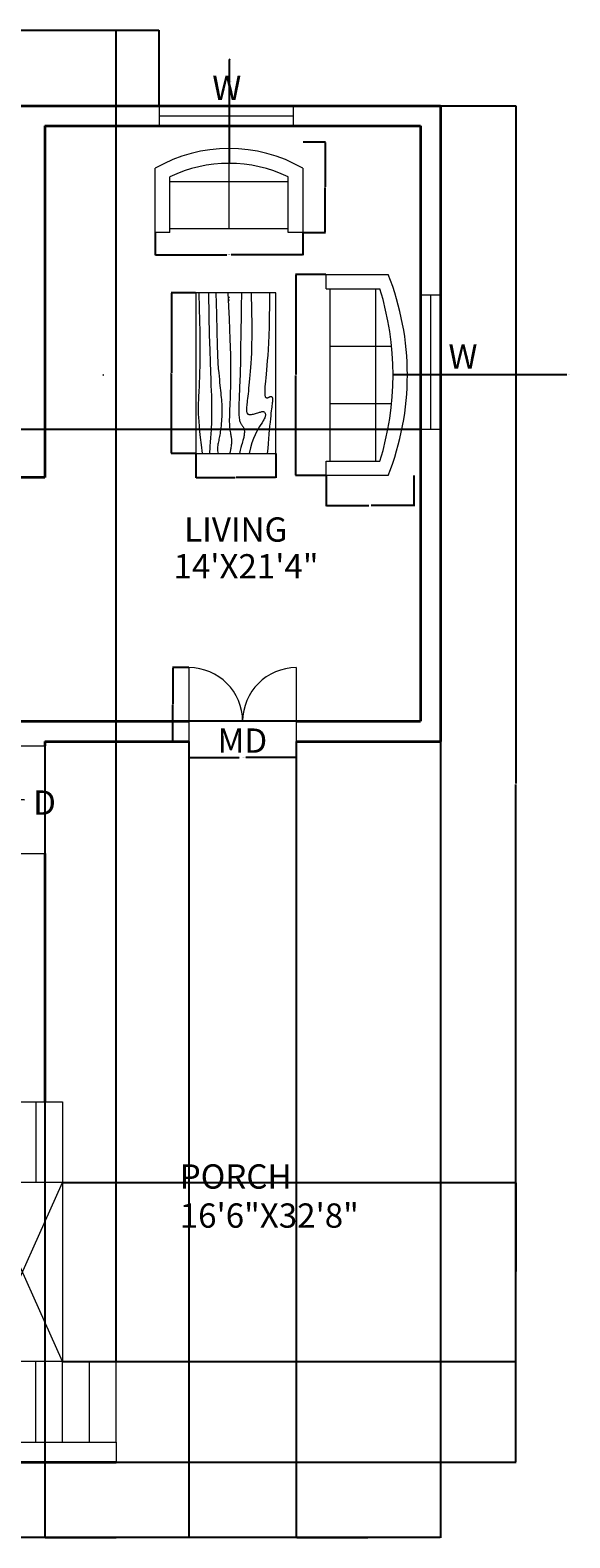
# Model space of a CAD drawing. Units: feet. Extents: x 1681 to 2398, y 1737 to 2411.
# Tile 4 of 4: x 2156 to 2398, y 1737 to 2411. Entities that reach past the tile are written whole.
import ezdxf

# ---------------------------------------------------------------- set-up
doc = ezdxf.new("R2010")
doc.units = ezdxf.units.FT
for name, color, linetype, lineweight in [('A-ANNO-DIMS', 2, 'Continuous', 18), ('A-ANNO-TEXT', 7, 'Continuous', 18), ('A-AREA-IDEN', 7, 'Continuous', 18), ('A-DOOR', 3, 'Continuous', 18), ('A-FLOR', 7, 'Continuous', 25), ('A-FLOR-STRS', 7, 'Continuous', 18), ('A-FURN', 8, 'Continuous', 13), ('A-GLAZ', 4, 'Continuous', 18), ('A-WALL', 7, 'Continuous', 35)]:
    doc.layers.add(name, color=color, linetype=linetype, lineweight=lineweight)
doc.styles.get("Standard").update_dxf_attribs({"font": 'arial.ttf'})
doc.dimstyles.get("Standard").update_dxf_attribs({"dimtxt": 0.18, "dimasz": 0.18, "dimexe": 0.18, "dimexo": 0.0625, "dimgap": 0.09, "dimtad": 0, "dimtih": 1, "dimtoh": 1, "dimdec": 4, "dimzin": 0, "dimdsep": 46, "dimtxsty": 'Standard', "dimcen": 0.09, "dimadec": 0, "dimazin": 0, "dimtfac": 1, "dimtdec": 4, "dimtofl": 0, "dimtmove": 0, "dimatfit": 3, "dimfxl": 1, "dimtolj": 1, "dimtzin": 0, "dimarcsym": 0})

# ---------------------------------------------------------------- blocks, each defined once
blk = doc.blocks.new('Sofa - Roundback 7 ft.')
for p, q in [((-36.000027, -34), (-36.000027, -11.4696)), ((-12.00002, -32.4421), (-12.00003, -6.5971)), ((11.99997, -32.4421), (11.99998, -6.5971)), ((35.99998, -34), (35.99998, -11.4696)), ((-35.999844, -13.3819), (35.9998, -13.3819)), ((-36.000027, -32.4421), (35.99998, -32.4421))]:
    blk.add_line(p, q)
for points in [[(-36.000027, -34), (-42.000027, -34), (-42.000027, -8)], [(41.99998, -8), (41.99998, -34), (35.99998, -34)]]:
    blk.add_lwpolyline(points)
for centre, radius, start, end in [((0, -114.25), 114.25, 68.43141, 111.5686), ((-0.00001, -127.1968), 121.1968, 72.72033, 107.2797)]:
    blk.add_arc(centre, radius, start, end)
blk = doc.blocks.new('Sofa - Roundback Loveseat 5 ft.')
for p, q in [((0, -32.44198), (0, -5.99998)), ((-24, -33.99998), (-24, -11.46958)), ((24.00004, -33.99998), (24.00004, -11.46958)), ((-23.9998, -13.38178), (23.99986, -13.38178)), ((-24, -32.44198), (24.00004, -32.44198))]:
    blk.add_line(p, q)
for points in [[(-24, -33.99998), (-30, -33.99998), (-30, -7.99998)], [(30.00004, -7.99998), (30.00004, -33.99998), (24.00004, -33.99998)]]:
    blk.add_lwpolyline(points)
for centre, radius, start, end in [((0, -60.24998), 60.24998, 60.13715, 119.8628), ((0, -61.38438), 55.38444, 64.32083, 115.6792)]:
    blk.add_arc(centre, radius, start, end)
blk = doc.blocks.new('Table - Rectangular Woodgrain 60 x 30 in.')
for p, q in [((0, 0), (0, -30)), ((60, 0), (0, 0)), ((60, -30), (60, 0)), ((0, -30), (60, -30))]:
    blk.add_line(p, q)
for points in [[(0, -2.4), (4.8155, -2.418), (9.0302, -2.4688), (12.709, -2.5477), (15.9167, -2.65), (18.7181, -2.7711), (21.1781, -2.9063), (23.3616, -3.0508), (25.3333, -3.2), (27.1477, -3.3495), (28.8172, -3.4958), (30.3437, -3.636), (31.7291, -3.7667), (32.9756, -3.8849), (34.0849, -3.9875), (35.059, -4.0714), (35.9, -4.1334), (36.6114, -4.1711), (37.2041, -4.1854), (37.6906, -4.1779), (38.0833, -4.15), (38.3948, -4.1034), (38.6375, -4.0396), (38.8239, -3.9602), (38.9666, -3.8667), (39.0764, -3.7608), (39.1573, -3.6448), (39.2116, -3.521), (39.2416, -3.3917), (39.2498, -3.2593), (39.2385, -3.1261), (39.21, -2.9944), (39.1666, -2.8667), (39.111, -2.7447), (39.0468, -2.6281), (38.978, -2.5163), (38.9083, -2.4083), (38.8418, -2.3035), (38.7823, -2.201), (38.7337, -2.1001), (38.7, -2), (38.6844, -1.9003), (38.6875, -1.8021), (38.7094, -1.707), (38.75, -1.6167), (38.8094, -1.5326), (38.8875, -1.4563), (38.9844, -1.3893), (39.1, -1.3333), (39.2351, -1.2896), (39.3937, -1.2583), (39.5804, -1.2396), (39.8, -1.2333), (40.057, -1.2396), (40.3562, -1.2583), (40.7023, -1.2896), (41.1, -1.3333), (41.5547, -1.3895), (42.0755, -1.4573), (42.6721, -1.5361), (43.3542, -1.625), (44.1316, -1.7233), (45.014, -1.8302), (46.0114, -1.9449), (47.1333, -2.0667), (48.3862, -2.1947), (49.7625, -2.3281), (51.2513, -2.4663), (52.8416, -2.6083), (54.5226, -2.7535), (56.2833, -2.9011), (58.1127, -3.0501), (60, -3.2)], [(0, -9.2), (6.5759, -9.0858), (11.9385, -9.0365), (16.2527, -9.0418), (19.6833, -9.0917), (22.3952, -9.1759), (24.5531, -9.2844), (26.322, -9.4069), (27.8666, -9.5333), (29.3241, -9.6553), (30.7203, -9.7719), (32.0532, -9.8837), (33.3208, -9.9917), (34.5213, -10.0965), (35.6526, -10.199), (36.7128, -10.2999), (37.7, -10.4), (38.6129, -10.4996), (39.4531, -10.5969), (40.223, -10.6895), (40.925, -10.775), (41.5613, -10.8512), (42.1344, -10.9156), (42.6465, -10.966), (43.1, -11), (43.4976, -11.0158), (43.8437, -11.0136), (44.143, -10.9942), (44.4, -10.9583), (44.6195, -10.9069), (44.8062, -10.8406), (44.9648, -10.7603), (45.1, -10.6667), (45.2155, -10.5598), (45.3114, -10.4365), (45.3871, -10.2929), (45.4416, -10.125), (45.4743, -9.929), (45.4844, -9.7011), (45.4709, -9.4371), (45.4333, -9.1333), (45.3716, -8.7883), (45.2896, -8.4104), (45.1919, -8.0107), (45.0833, -7.6), (44.9685, -7.1893), (44.8521, -6.7896), (44.7388, -6.4117), (44.6333, -6.0667), (44.54, -5.7628), (44.4614, -5.4979), (44.4001, -5.2675), (44.3583, -5.0667), (44.3384, -4.8909), (44.3427, -4.7354), (44.3736, -4.5956), (44.4333, -4.4667), (44.5236, -4.3453), (44.6427, -4.2333), (44.7884, -4.1339), (44.9583, -4.05), (45.1501, -3.9849), (45.3614, -3.9417), (45.59, -3.9234), (45.8333, -3.9333), (46.0915, -3.9749), (46.3734, -4.0531), (46.6906, -4.1736), (47.0542, -4.3417), (47.4756, -4.5629), (47.9661, -4.8427), (48.5372, -5.1866), (49.2, -5.6), (49.9676, -6.0844), (50.8594, -6.625), (51.8965, -7.2031), (53.1, -7.8), (54.491, -8.3969), (56.0906, -8.975), (57.9199, -9.5156), (60, -10)], [(0, -12.8), (5.1847, -12.9322), (9.6213, -13.0323), (13.3963, -13.1059), (16.5958, -13.1583), (19.3063, -13.1952), (21.614, -13.2219), (23.6054, -13.2439), (25.3666, -13.2667), (26.9728, -13.2947), (28.4531, -13.3281), (29.8256, -13.3663), (31.1083, -13.4083), (32.3191, -13.4535), (33.476, -13.501), (34.597, -13.5501), (35.7, -13.6), (36.7984, -13.6497), (37.8875, -13.6979), (38.9578, -13.743), (40, -13.7833), (41.0047, -13.8174), (41.9625, -13.8438), (42.864, -13.8607), (43.7, -13.8667), (44.4631, -13.8604), (45.1552, -13.8417), (45.7801, -13.8104), (46.3416, -13.7667), (46.8439, -13.7104), (47.2906, -13.6417), (47.6858, -13.5604), (48.0333, -13.4667), (48.3375, -13.3608), (48.6042, -13.2448), (48.8396, -13.121), (49.05, -12.9917), (49.2417, -12.8593), (49.4208, -12.7261), (49.5937, -12.5944), (49.7667, -12.4667), (49.9452, -12.3451), (50.1323, -12.2313), (50.3303, -12.1268), (50.5416, -12.0333), (50.7686, -11.9524), (51.0135, -11.8854), (51.2788, -11.8341), (51.5666, -11.8), (51.8785, -11.7843), (52.2116, -11.7865), (52.562, -11.8059), (52.926, -11.8417), (53.2998, -11.8931), (53.6795, -11.9594), (54.0614, -12.0397), (54.4416, -12.1333), (54.8223, -12.2401), (55.2293, -12.3625), (55.6942, -12.5037), (56.2489, -12.6667), (56.9251, -12.8547), (57.7545, -13.0708), (58.7689, -13.3182), (60, -13.6)], [(0, -18), (5.124, -17.7273), (9.6609, -17.5057), (13.6705, -17.3303), (17.2125, -17.1958), (20.3467, -17.0973), (23.1328, -17.0297), (25.6307, -16.9878), (27.9, -16.9667), (29.9928, -16.9617), (31.9302, -16.9703), (33.7254, -16.9907), (35.3917, -17.0208), (36.9423, -17.0588), (38.3906, -17.1026), (39.7499, -17.1503), (41.0333, -17.2), (42.2519, -17.2496), (43.4073, -17.2969), (44.4986, -17.3395), (45.525, -17.375), (46.4858, -17.4012), (47.3802, -17.4156), (48.2074, -17.416), (48.9667, -17.4), (49.6583, -17.3662), (50.2872, -17.3167), (50.8595, -17.2547), (51.3812, -17.1833), (51.8584, -17.1057), (52.2971, -17.025), (52.7034, -16.9443), (53.0833, -16.8667), (53.443, -16.7951), (53.789, -16.7313), (54.128, -16.6768), (54.4666, -16.6334), (54.8115, -16.6024), (55.1693, -16.5854), (55.5465, -16.5841), (55.95, -16.6), (56.3828, -16.6337), (56.8346, -16.6823), (57.2915, -16.7418), (57.7396, -16.8084), (58.165, -16.878), (58.5539, -16.9469), (58.8924, -17.0111), (59.1666, -17.0667), (59.3679, -17.1107), (59.5078, -17.1438), (59.6032, -17.1675), (59.6708, -17.1833), (59.7275, -17.193), (59.7901, -17.1979), (59.8753, -17.1998), (60, -17.2)], [(0, -22.4), (8.0098, -22.2501), (14.4094, -22.1011), (19.4168, -21.9535), (23.25, -21.8083), (26.1269, -21.6663), (28.2656, -21.5281), (29.884, -21.3947), (31.2, -21.2667), (32.3967, -21.1448), (33.5172, -21.0292), (34.5697, -20.9198), (35.5625, -20.8167), (36.5037, -20.7198), (37.4015, -20.6292), (38.2642, -20.5448), (39.1, -20.4667), (39.9164, -20.3951), (40.7187, -20.3313), (41.5117, -20.2768), (42.3, -20.2333), (43.0883, -20.2024), (43.8812, -20.1854), (44.6836, -20.1841), (45.5, -20.2), (46.3328, -20.234), (47.1747, -20.2844), (48.0163, -20.3488), (48.8479, -20.425), (49.66, -20.5106), (50.4429, -20.6031), (51.1872, -20.7004), (51.8833, -20.8), (52.5246, -20.8999), (53.1166, -20.9995), (53.6681, -21.0983), (54.1875, -21.1958), (54.6834, -21.2919), (55.1646, -21.3859), (55.6394, -21.4777), (56.1167, -21.5667), (56.6028, -21.6515), (57.0961, -21.7266), (57.5929, -21.7852), (58.0896, -21.8208), (58.5823, -21.8268), (59.0674, -21.7964), (59.5412, -21.723), (60, -21.6)], [(0, -25.2), (8.6355, -25.0504), (15.7026, -24.9031), (21.4049, -24.7606), (25.9458, -24.625), (29.529, -24.4988), (32.3578, -24.3844), (34.6359, -24.284), (36.5667, -24.2), (38.3213, -24.1341), (39.9417, -24.0854), (41.437, -24.0523), (42.8167, -24.0333), (44.0901, -24.0268), (45.2667, -24.0313), (46.3557, -24.0451), (47.3667, -24.0667), (48.309, -24.0947), (49.1928, -24.1287), (50.0284, -24.168), (50.826, -24.2125), (51.5959, -24.2617), (52.3483, -24.3151), (53.0935, -24.3725), (53.8417, -24.4334), (54.6009, -24.497), (55.3699, -24.561), (56.1454, -24.6226), (56.9239, -24.6792), (57.7021, -24.7279), (58.4764, -24.7662), (59.2435, -24.7911), (60, -24.8)], [(0, -28.8), (5.6867, -28.6681), (10.45, -28.5698), (14.407, -28.5012), (17.675, -28.4584), (20.3711, -28.4374), (22.6125, -28.4344), (24.5164, -28.4455), (26.2, -28.4667), (27.762, -28.4947), (29.2276, -28.5281), (30.6033, -28.5663), (31.8958, -28.6084), (33.1118, -28.6535), (34.2578, -28.7011), (35.3405, -28.7501), (36.3666, -28.8), (37.3443, -28.8497), (38.288, -28.8974), (39.2137, -28.9412), (40.1375, -28.9792), (41.0753, -29.0093), (42.0432, -29.0297), (43.0572, -29.0384), (44.1333, -29.0333), (45.2936, -29.0114), (46.5843, -28.9641), (48.0579, -28.8816), (49.7666, -28.7542), (51.7629, -28.5721), (54.0989, -28.3255), (56.8272, -28.0048), (60, -27.6)]]:
    blk.add_lwpolyline(points)
blk = doc.blocks.new('DOOR-DOUBLE-SWING')
for p, q in [((0, 48), (33, 48)), ((0, 0), (33, 0))]:
    blk.add_line(p, q)
for centre, start, end in [((24, 48), 180, 270), ((24, 0), 90, 180)]:
    blk.add_arc(centre, 24, start, end)
blk = doc.blocks.new('WINDOW-STANDARD')
for p, q in [((0, 9), (0, 0)), ((60, 9), (60, 0)), ((0, 4.5), (60, 4.5))]:
    blk.add_line(p, q)
blk = doc.blocks.new('*D24')
at = {"layer": 'A-ANNO-DIMS', "color": 0, "lineweight": -2, "transparency": 16777216}
for p, q in [((2288.49, 2301.7), (2274.9, 2301.7)), ((2275.08, 2301.52), (2275.08, 2256.98)), ((2275.08, 2212.07), (2275.08, 2256.61)), ((2288.49, 2211.89), (2274.9, 2211.89))]:
    blk.add_line(p, q, dxfattribs=at)
at = {"layer": 'A-ANNO-DIMS', "color": 0, "transparency": 16777216}
for points in [[(2275.05, 2301.52), (2275.11, 2301.52), (2275.08, 2301.7)], [(2275.05, 2212.07), (2275.11, 2212.07), (2275.08, 2211.89)]]:
    blk.add_solid(points, dxfattribs=at)
at = {"layer": 'Defpoints', "color": 0, "transparency": 16777216}
for p in [(2288.55, 2301.7), (2275.08, 2211.89), (2288.55, 2211.89)]:
    blk.add_point(p, dxfattribs=at)
at = {"layer": 'A-ANNO-DIMS', "color": 0, "transparency": 16777216, "insert": (2275.08, 2256.8), "char_height": 0.18, "attachment_point": 5}
blk.add_mtext('\\A1;SOFA 90 TYP.', dxfattribs=at)
blk = doc.blocks.new('*D25')
at = {"layer": 'A-ANNO-DIMS', "color": 0, "lineweight": -2, "transparency": 16777216}
for p, q in [((2288.55, 2211.83), (2288.55, 2198.24)), ((2327.75, 2211.83), (2327.75, 2198.24)), ((2288.73, 2198.42), (2307.62, 2198.42)), ((2327.57, 2198.42), (2308.68, 2198.42))]:
    blk.add_line(p, q, dxfattribs=at)
at = {"layer": 'A-ANNO-DIMS', "color": 0, "transparency": 16777216}
for points in [[(2288.73, 2198.45), (2288.73, 2198.39), (2288.55, 2198.42)], [(2327.57, 2198.45), (2327.57, 2198.39), (2327.75, 2198.42)]]:
    blk.add_solid(points, dxfattribs=at)
at = {"layer": 'Defpoints', "color": 0, "transparency": 16777216}
for p in [(2288.55, 2211.89), (2327.75, 2211.89), (2327.75, 2198.42)]:
    blk.add_point(p, dxfattribs=at)
at = {"layer": 'A-ANNO-DIMS', "color": 0, "transparency": 16777216, "insert": (2308.15, 2198.42), "char_height": 0.18, "attachment_point": 5}
blk.add_mtext('\\A1;39 TYP.', dxfattribs=at)
blk = doc.blocks.new('*D26')
at = {"layer": 'A-ANNO-DIMS', "color": 0, "lineweight": -2, "transparency": 16777216}
for p, q in [((2230.17, 2293.48), (2219.29, 2293.48)), ((2219.47, 2293.3), (2219.47, 2257.79)), ((2219.47, 2221.92), (2219.47, 2257.43)), ((2230.17, 2221.74), (2219.29, 2221.74))]:
    blk.add_line(p, q, dxfattribs=at)
at = {"layer": 'A-ANNO-DIMS', "color": 0, "transparency": 16777216}
for points in [[(2219.44, 2293.3), (2219.5, 2293.3), (2219.47, 2293.48)], [(2219.44, 2221.92), (2219.5, 2221.92), (2219.47, 2221.74)]]:
    blk.add_solid(points, dxfattribs=at)
at = {"layer": 'Defpoints', "color": 0, "transparency": 16777216}
for p in [(2230.23, 2293.48), (2219.47, 2221.74), (2230.23, 2221.74)]:
    blk.add_point(p, dxfattribs=at)
at = {"layer": 'A-ANNO-DIMS', "color": 0, "transparency": 16777216, "insert": (2219.47, 2257.61), "char_height": 0.18, "attachment_point": 5}
blk.add_mtext('\\A1;COFFEE TABLE 72', dxfattribs=at)
blk = doc.blocks.new('*D27')
at = {"layer": 'A-ANNO-DIMS', "color": 0, "lineweight": -2, "transparency": 16777216}
for p, q in [((2230.23, 2221.68), (2230.23, 2210.8)), ((2266.1, 2221.68), (2266.1, 2210.8)), ((2230.41, 2210.98), (2247.94, 2210.98)), ((2265.92, 2210.98), (2248.38, 2210.98))]:
    blk.add_line(p, q, dxfattribs=at)
at = {"layer": 'A-ANNO-DIMS', "color": 0, "transparency": 16777216}
for points in [[(2230.41, 2211.01), (2230.41, 2210.95), (2230.23, 2210.98)], [(2265.92, 2211.01), (2265.92, 2210.95), (2266.1, 2210.98)]]:
    blk.add_solid(points, dxfattribs=at)
at = {"layer": 'Defpoints', "color": 0, "transparency": 16777216}
for p in [(2230.23, 2221.74), (2266.1, 2221.74), (2266.1, 2210.98)]:
    blk.add_point(p, dxfattribs=at)
at = {"layer": 'A-ANNO-DIMS', "color": 0, "transparency": 16777216, "insert": (2248.16, 2210.98), "char_height": 0.18, "attachment_point": 5}
blk.add_mtext('\\A1;36', dxfattribs=at)
blk = doc.blocks.new('*D30')
at = {"layer": 'A-ANNO-DIMS', "color": 0, "lineweight": -2, "transparency": 16777216}
for p, q in [((2227.24, 2092.99), (2227.24, 2085.67)), ((2275.24, 2092.99), (2275.24, 2085.67)), ((2227.42, 2085.85), (2249.75, 2085.85)), ((2275.06, 2085.85), (2252.73, 2085.85))]:
    blk.add_line(p, q, dxfattribs=at)
at = {"layer": 'A-ANNO-DIMS', "color": 0, "transparency": 16777216}
for points in [[(2227.42, 2085.88), (2227.42, 2085.82), (2227.24, 2085.85)], [(2275.06, 2085.88), (2275.06, 2085.82), (2275.24, 2085.85)]]:
    blk.add_solid(points, dxfattribs=at)
at = {"layer": 'Defpoints', "color": 0, "transparency": 16777216}
for p in [(2227.24, 2093.05), (2275.24, 2093.05), (2275.24, 2085.85)]:
    blk.add_point(p, dxfattribs=at)
at = {"layer": 'A-ANNO-DIMS', "color": 0, "transparency": 16777216, "insert": (2251.24, 2085.85), "char_height": 0.18, "attachment_point": 5}
blk.add_mtext('\\A1;DOUBLE DOOR 48 TYP.', dxfattribs=at)
blk = doc.blocks.new('*D31')
at = {"layer": 'A-ANNO-DIMS', "color": 0, "lineweight": -2, "transparency": 16777216}
for p, q in [((2227.18, 2126.05), (2219.86, 2126.05)), ((2220.04, 2125.87), (2220.04, 2109.73)), ((2220.04, 2093.23), (2220.04, 2109.37)), ((2227.18, 2093.05), (2219.86, 2093.05))]:
    blk.add_line(p, q, dxfattribs=at)
at = {"layer": 'A-ANNO-DIMS', "color": 0, "transparency": 16777216}
for points in [[(2220.01, 2125.87), (2220.07, 2125.87), (2220.04, 2126.05)], [(2220.01, 2093.23), (2220.07, 2093.23), (2220.04, 2093.05)]]:
    blk.add_solid(points, dxfattribs=at)
at = {"layer": 'Defpoints', "color": 0, "transparency": 16777216}
for p in [(2227.24, 2126.05), (2220.04, 2093.05), (2227.24, 2093.05)]:
    blk.add_point(p, dxfattribs=at)
at = {"layer": 'A-ANNO-DIMS', "color": 0, "transparency": 16777216, "insert": (2220.04, 2109.55), "char_height": 0.18, "attachment_point": 5}
blk.add_mtext('\\A1;33 TYP.', dxfattribs=at)
blk = doc.blocks.new('*D38')
at = {"layer": 'A-ANNO-DIMS', "color": 0, "lineweight": -2, "transparency": 16777216}
for p, q in [((2212.06, 2320.38), (2212.06, 2310.34)), ((2278.22, 2320.38), (2278.22, 2310.34)), ((2212.24, 2310.52), (2244.22, 2310.52)), ((2278.04, 2310.52), (2246.05, 2310.52))]:
    blk.add_line(p, q, dxfattribs=at)
at = {"layer": 'A-ANNO-DIMS', "color": 0, "transparency": 16777216}
for points in [[(2212.24, 2310.55), (2212.24, 2310.49), (2212.06, 2310.52)], [(2278.04, 2310.55), (2278.04, 2310.49), (2278.22, 2310.52)]]:
    blk.add_solid(points, dxfattribs=at)
at = {"layer": 'Defpoints', "color": 0, "transparency": 16777216}
for p in [(2212.06, 2320.44), (2278.22, 2320.44), (2278.22, 2310.52)]:
    blk.add_point(p, dxfattribs=at)
at = {"layer": 'A-ANNO-DIMS', "color": 0, "transparency": 16777216, "insert": (2245.14, 2310.52), "char_height": 0.18, "attachment_point": 5}
blk.add_mtext('\\A1;LOVESEAT 66', dxfattribs=at)
blk = doc.blocks.new('*D39')
at = {"layer": 'A-ANNO-DIMS', "color": 0, "lineweight": -2, "transparency": 16777216}
for p, q in [((2278.28, 2360.87), (2288.32, 2360.87)), ((2288.14, 2360.69), (2288.14, 2340.84)), ((2288.14, 2320.62), (2288.14, 2340.48)), ((2278.28, 2320.44), (2288.32, 2320.44))]:
    blk.add_line(p, q, dxfattribs=at)
at = {"layer": 'A-ANNO-DIMS', "color": 0, "transparency": 16777216}
for points in [[(2288.11, 2360.69), (2288.17, 2360.69), (2288.14, 2360.87)], [(2288.11, 2320.62), (2288.17, 2320.62), (2288.14, 2320.44)]]:
    blk.add_solid(points, dxfattribs=at)
at = {"layer": 'Defpoints', "color": 0, "transparency": 16777216}
for p in [(2278.22, 2360.87), (2288.14, 2360.87), (2278.22, 2320.44)]:
    blk.add_point(p, dxfattribs=at)
at = {"layer": 'A-ANNO-DIMS', "color": 0, "transparency": 16777216, "insert": (2288.14, 2340.66), "char_height": 0.18, "attachment_point": 5}
blk.add_mtext('\\A1;40', dxfattribs=at)
blk = doc.blocks.new('*D40')
at = {"layer": 'A-ANNO-DIMS', "color": 0, "lineweight": -2, "transparency": 16777216}
for p, q in [((1714.74, 1770.99), (1714.74, 1737.27)), ((2339.74, 1770.99), (2339.74, 1737.27)), ((1714.92, 1737.45), (2026.95, 1737.45)), ((2339.56, 1737.45), (2027.53, 1737.45))]:
    blk.add_line(p, q, dxfattribs=at)
at = {"layer": 'A-ANNO-DIMS', "color": 0, "transparency": 16777216}
for points in [[(1714.92, 1737.48), (1714.92, 1737.42), (1714.74, 1737.45)], [(2339.56, 1737.48), (2339.56, 1737.42), (2339.74, 1737.45)]]:
    blk.add_solid(points, dxfattribs=at)
at = {"layer": 'Defpoints', "color": 0, "transparency": 16777216}
for p in [(1714.74, 1771.05), (2339.74, 1771.05), (2339.74, 1737.45)]:
    blk.add_point(p, dxfattribs=at)
at = {"layer": 'A-ANNO-DIMS', "color": 0, "transparency": 16777216, "insert": (2027.24, 1737.45), "char_height": 0.18, "attachment_point": 5}
blk.add_mtext('\\A1;625', dxfattribs=at)
blk = doc.blocks.new('*D41')
at = {"layer": 'A-ANNO-DIMS', "color": 0, "lineweight": -2, "transparency": 16777216}
for p, q in [((2339.8, 2377.05), (2373.52, 2377.05)), ((2373.34, 2376.87), (2373.34, 2074.23)), ((2373.34, 1771.23), (2373.34, 2073.87)), ((2339.8, 1771.05), (2373.52, 1771.05))]:
    blk.add_line(p, q, dxfattribs=at)
at = {"layer": 'A-ANNO-DIMS', "color": 0, "transparency": 16777216}
for points in [[(2373.31, 2376.87), (2373.37, 2376.87), (2373.34, 2377.05)], [(2373.31, 1771.23), (2373.37, 1771.23), (2373.34, 1771.05)]]:
    blk.add_solid(points, dxfattribs=at)
at = {"layer": 'Defpoints', "color": 0, "transparency": 16777216}
for p in [(2339.74, 2377.05), (2339.74, 1771.05), (2373.34, 1771.05)]:
    blk.add_point(p, dxfattribs=at)
at = {"layer": 'A-ANNO-DIMS', "color": 0, "transparency": 16777216, "insert": (2373.34, 2074.05), "char_height": 0.18, "attachment_point": 5}
blk.add_mtext('\\A1;606', dxfattribs=at)
blk = doc.blocks.new('*D45')
at = {"layer": 'A-ANNO-DIMS', "color": 0, "lineweight": -2, "transparency": 16777216}
for p, q in [((2042.03, 2377.11), (2042.03, 2410.83)), ((2042.21, 2410.65), (2127.5, 2410.65)), ((2213.71, 2410.65), (2128.42, 2410.65)), ((2213.89, 2377.11), (2213.89, 2410.83))]:
    blk.add_line(p, q, dxfattribs=at)
at = {"layer": 'A-ANNO-DIMS', "color": 0, "transparency": 16777216}
for points in [[(2042.21, 2410.68), (2042.21, 2410.62), (2042.03, 2410.65)], [(2213.71, 2410.68), (2213.71, 2410.62), (2213.89, 2410.65)]]:
    blk.add_solid(points, dxfattribs=at)
at = {"layer": 'Defpoints', "color": 0, "transparency": 16777216}
for p in [(2213.89, 2410.65), (2042.03, 2377.05), (2213.89, 2377.05)]:
    blk.add_point(p, dxfattribs=at)
at = {"layer": 'A-ANNO-DIMS', "color": 0, "transparency": 16777216, "insert": (2127.96, 2410.65), "char_height": 0.18, "attachment_point": 5}
blk.add_mtext('\\A1;171.85', dxfattribs=at)
blk = doc.blocks.new('*D50')
at = {"layer": 'A-ANNO-DIMS', "color": 0, "lineweight": -2, "transparency": 16777216}
for p, q in [((2330.68, 2232.39), (1680.96, 2232.39)), ((1681.14, 2232.21), (1681.14, 2167.4)), ((1681.14, 2102.23), (1681.14, 2167.04)), ((2330.68, 2102.05), (1680.96, 2102.05))]:
    blk.add_line(p, q, dxfattribs=at)
at = {"layer": 'A-ANNO-DIMS', "color": 0, "transparency": 16777216}
for points in [[(1681.11, 2232.21), (1681.17, 2232.21), (1681.14, 2232.39)], [(1681.11, 2102.23), (1681.17, 2102.23), (1681.14, 2102.05)]]:
    blk.add_solid(points, dxfattribs=at)
at = {"layer": 'Defpoints', "color": 0, "transparency": 16777216}
for p in [(1681.14, 2232.39), (2330.74, 2232.39), (2330.74, 2102.05)]:
    blk.add_point(p, dxfattribs=at)
at = {"layer": 'A-ANNO-DIMS', "color": 0, "transparency": 16777216, "insert": (1681.14, 2167.22), "char_height": 0.18, "attachment_point": 5}
blk.add_mtext('\\A1;130.34', dxfattribs=at)
blk = doc.blocks.new('*D53')
at = {"layer": 'A-ANNO-DIMS', "color": 0, "lineweight": -2, "transparency": 16777216}
for p, q in [((2098.74, 1816.11), (2098.74, 2410.83)), ((2098.92, 2410.65), (2146.52, 2410.65)), ((2194.56, 2410.65), (2146.96, 2410.65)), ((2194.74, 1816.11), (2194.74, 2410.83))]:
    blk.add_line(p, q, dxfattribs=at)
at = {"layer": 'A-ANNO-DIMS', "color": 0, "transparency": 16777216}
for points in [[(2098.92, 2410.68), (2098.92, 2410.62), (2098.74, 2410.65)], [(2194.56, 2410.68), (2194.56, 2410.62), (2194.74, 2410.65)]]:
    blk.add_solid(points, dxfattribs=at)
at = {"layer": 'Defpoints', "color": 0, "transparency": 16777216}
for p in [(2194.74, 2410.65), (2098.74, 1816.05), (2194.74, 1816.05)]:
    blk.add_point(p, dxfattribs=at)
at = {"layer": 'A-ANNO-DIMS', "color": 0, "transparency": 16777216, "insert": (2146.74, 2410.65), "char_height": 0.18, "attachment_point": 5}
blk.add_mtext('\\A1;96', dxfattribs=at)
blk = doc.blocks.new('*D54')
at = {"layer": 'A-ANNO-DIMS', "color": 0, "lineweight": -2, "transparency": 16777216}
for p, q in [((2170.8, 1896.05), (2373.52, 1896.05)), ((2373.34, 1895.87), (2373.34, 1856.23)), ((2373.34, 1816.23), (2373.34, 1855.87)), ((2170.8, 1816.05), (2373.52, 1816.05))]:
    blk.add_line(p, q, dxfattribs=at)
at = {"layer": 'A-ANNO-DIMS', "color": 0, "transparency": 16777216}
for points in [[(2373.31, 1895.87), (2373.37, 1895.87), (2373.34, 1896.05)], [(2373.31, 1816.23), (2373.37, 1816.23), (2373.34, 1816.05)]]:
    blk.add_solid(points, dxfattribs=at)
at = {"layer": 'Defpoints', "color": 0, "transparency": 16777216}
for p in [(2170.74, 1896.05), (2170.74, 1816.05), (2373.34, 1816.05)]:
    blk.add_point(p, dxfattribs=at)
at = {"layer": 'A-ANNO-DIMS', "color": 0, "transparency": 16777216, "insert": (2373.34, 1856.05), "char_height": 0.18, "attachment_point": 5}
blk.add_mtext('\\A1;80', dxfattribs=at)
blk = doc.blocks.new('*D56')
at = {"layer": 'A-ANNO-DIMS', "color": 0, "lineweight": -2, "transparency": 16777216}
for p, q in [((2275.24, 2092.99), (2275.24, 1737.27)), ((2339.74, 2092.99), (2339.74, 1737.27)), ((2275.42, 1737.45), (2307.17, 1737.45)), ((2339.56, 1737.45), (2307.82, 1737.45))]:
    blk.add_line(p, q, dxfattribs=at)
at = {"layer": 'A-ANNO-DIMS', "color": 0, "transparency": 16777216}
for points in [[(2275.42, 1737.48), (2275.42, 1737.42), (2275.24, 1737.45)], [(2339.56, 1737.48), (2339.56, 1737.42), (2339.74, 1737.45)]]:
    blk.add_solid(points, dxfattribs=at)
at = {"layer": 'Defpoints', "color": 0, "transparency": 16777216}
for p in [(2275.24, 2093.05), (2339.74, 2093.05), (2339.74, 1737.45)]:
    blk.add_point(p, dxfattribs=at)
at = {"layer": 'A-ANNO-DIMS', "color": 0, "transparency": 16777216, "insert": (2307.49, 1737.45), "char_height": 0.18, "attachment_point": 5}
blk.add_mtext('\\A1;64.5', dxfattribs=at)
blk = doc.blocks.new('*D61')
at = {"layer": 'A-ANNO-DIMS', "color": 0, "lineweight": -2, "transparency": 16777216}
for p, q in [((2162.74, 2092.99), (2162.74, 1737.27)), ((2227.24, 2092.99), (2227.24, 1737.27)), ((2162.92, 1737.45), (2194.67, 1737.45)), ((2227.06, 1737.45), (2195.32, 1737.45))]:
    blk.add_line(p, q, dxfattribs=at)
at = {"layer": 'A-ANNO-DIMS', "color": 0, "transparency": 16777216}
for points in [[(2162.92, 1737.48), (2162.92, 1737.42), (2162.74, 1737.45)], [(2227.06, 1737.48), (2227.06, 1737.42), (2227.24, 1737.45)]]:
    blk.add_solid(points, dxfattribs=at)
at = {"layer": 'Defpoints', "color": 0, "transparency": 16777216}
for p in [(2162.74, 2093.05), (2227.24, 2093.05), (2227.24, 1737.45)]:
    blk.add_point(p, dxfattribs=at)
at = {"layer": 'A-ANNO-DIMS', "color": 0, "transparency": 16777216, "insert": (2194.99, 1737.45), "char_height": 0.18, "attachment_point": 5}
blk.add_mtext('\\A1;64.5', dxfattribs=at)
blk = doc.blocks.new('*D64')
at = {"layer": 'A-ANNO-DIMS', "color": 0, "lineweight": -2, "transparency": 16777216}
for p, q in [((2188.82, 2256.8), (2189, 2256.8)), ((2188.91, 2256.71), (2188.91, 2256.89)), ((2396.22, 2256.79), (2318.66, 2256.79))]:
    blk.add_line(p, q, dxfattribs=at)
at = {"layer": 'A-ANNO-DIMS', "color": 0, "transparency": 16777216}
blk.add_solid([(2318.66, 2256.82), (2318.66, 2256.76), (2318.48, 2256.79)], dxfattribs=at)
at = {"layer": 'Defpoints', "color": 0, "transparency": 16777216}
for p in [(2188.91, 2256.8), (2318.48, 2256.79)]:
    blk.add_point(p, dxfattribs=at)
at = {"layer": 'A-ANNO-DIMS', "color": 0, "transparency": 16777216, "insert": (2396.97, 2256.79), "char_height": 0.18, "attachment_point": 5}
blk.add_mtext('\\A1;2X R129.57', dxfattribs=at)
blk = doc.blocks.new('*D66')
at = {"layer": 'A-ANNO-DIMS', "color": 0, "lineweight": -2, "transparency": 16777216}
for p, q in [((2245.32, 2397.79), (2245.14, 2397.79)), ((2245.14, 2397.79), (2245.14, 2358.11)), ((2245.05, 2291.5), (2245.23, 2291.5)), ((2245.14, 2291.41), (2245.14, 2291.59))]:
    blk.add_line(p, q, dxfattribs=at)
at = {"layer": 'A-ANNO-DIMS', "color": 0, "transparency": 16777216}
blk.add_solid([(2245.11, 2358.11), (2245.17, 2358.11), (2245.14, 2357.93)], dxfattribs=at)
at = {"layer": 'Defpoints', "color": 0, "transparency": 16777216}
for p in [(2245.14, 2357.93), (2245.14, 2291.5)]:
    blk.add_point(p, dxfattribs=at)
at = {"layer": 'A-ANNO-DIMS', "color": 0, "transparency": 16777216, "insert": (2245.8, 2397.79), "char_height": 0.18, "attachment_point": 5}
blk.add_mtext('\\A1;R66.44', dxfattribs=at)
blk = doc.blocks.new('*D67')
at = {"layer": 'A-ANNO-DIMS', "color": 0, "lineweight": -2, "transparency": 16777216}
for p, q in [((2245.32, 2387.96), (2245.14, 2387.96)), ((2245.14, 2387.96), (2245.14, 2351.5)), ((2245.05, 2290.25), (2245.23, 2290.25)), ((2245.14, 2290.16), (2245.14, 2290.34))]:
    blk.add_line(p, q, dxfattribs=at)
at = {"layer": 'A-ANNO-DIMS', "color": 0, "transparency": 16777216}
blk.add_solid([(2245.11, 2351.5), (2245.17, 2351.5), (2245.14, 2351.32)], dxfattribs=at)
at = {"layer": 'Defpoints', "color": 0, "transparency": 16777216}
for p in [(2245.14, 2351.32), (2245.14, 2290.25)]:
    blk.add_point(p, dxfattribs=at)
at = {"layer": 'A-ANNO-DIMS', "color": 0, "transparency": 16777216, "insert": (2245.8, 2387.96), "char_height": 0.18, "attachment_point": 5}
blk.add_mtext('\\A1;R61.07', dxfattribs=at)

msp = doc.modelspace()

# ---------------------------------------------------------------- linework, layer by layer
at = {"layer": 'A-FLOR'}
for p in [(2339.7402, 2093.0485), (1965.7402, 1771.0485)]:
    msp.add_line(p, (2339.7402, 1771.0485), dxfattribs=at)
at = {"layer": 'A-FLOR-STRS'}
for p, q in [((2134.7402, 1932.0485), (2170.7402, 1932.0485)), ((2158.7402, 1932.0485), (2158.7402, 1896.0485)), ((2170.7402, 1932.0485), (2170.7402, 1816.0485)), ((2170.7402, 1896.0485), (2134.7402, 1896.0485)), ((2170.7402, 1816.0485), (2134.7402, 1896.0485)), ((2134.7402, 1816.0485), (2170.7402, 1896.0485)), ((2194.7402, 1816.0485), (2134.7402, 1816.0485)), ((2158.7402, 1780.0485), (2158.7402, 1816.0485)), ((2170.7402, 1780.0485), (2170.7402, 1816.0485)), ((2182.7402, 1780.0485), (2182.7402, 1816.0485)), ((2194.7402, 1780.0485), (2194.7402, 1816.0485)), ((2134.7402, 1780.0485), (2194.7402, 1780.0485)), ((2194.7402, 1780.0485), (2194.7402, 1771.0485))]:
    msp.add_line(p, q, dxfattribs=at)
at = {"layer": 'A-WALL'}
for p, q in [((1714.7402, 2377.0485), (2339.7402, 2377.0485)), ((1916.7402, 2377.0485), (2339.7402, 2377.0485)), ((2162.7402, 2377.0485), (2339.7402, 2377.0485)), ((2339.7402, 2377.0485), (2339.7402, 2093.0485)), ((2162.7402, 2368.0485), (2162.7402, 2211.0485)), ((2162.7402, 2368.0485), (2330.7402, 2368.0485)), ((2330.7402, 2368.0485), (2330.7402, 2102.0485)), ((2162.7402, 2211.0485), (2023.7402, 2211.0485)), ((2137.7992, 2102.0485), (2227.2402, 2102.0485)), ((2275.2402, 2102.0485), (2330.7402, 2102.0485)), ((2162.7402, 2093.0485), (2162.7402, 2091.0485)), ((2162.7402, 2093.0485), (2227.2402, 2093.0485)), ((2275.2402, 2093.0485), (2339.7402, 2093.0485)), ((2162.7402, 2043.0485), (2162.7402, 1932.0485)), ((1714.7402, 1771.0485), (2194.7402, 1771.0485)), ((1880.7402, 1771.0485), (2194.7402, 1771.0485))]:
    msp.add_line(p, q, dxfattribs=at)

# ---------------------------------------------------------------- block references
at = {"layer": 'A-DOOR', "rotation": 270}
msp.add_blockref('DOOR-DOUBLE-SWING', (2227.2402, 2126.0485), dxfattribs=at)
at = {"layer": 'A-DOOR'}
msp.add_blockref('DOOR-DOUBLE-SWING', (2129.7402, 2043.0485), dxfattribs=at)
at = {"layer": 'A-FURN', "xscale": 1.102672576949214, "yscale": 1.102672576949214, "zscale": 1.102672576949214}
msp.add_blockref('Sofa - Roundback Loveseat 5 ft.', (2245.1371, 2357.9328), dxfattribs=at)
at = {"layer": 'A-FURN', "rotation": 270}
for name, p, xscale, yscale, zscale in [('Sofa - Roundback 7 ft.', (2324.8978, 2256.7954), 1.069080003544779, 1.069080003544779, 1.069080003544779), ('Table - Rectangular Woodgrain 60 x 30 in.', (2266.0962, 2293.4787), 1.195571873493857, 1.195571873493857, 1.195571873493857)]:
    msp.add_blockref(name, p, dxfattribs=dict(at, xscale=xscale, yscale=yscale, zscale=zscale))
at = {"layer": 'A-GLAZ'}
msp.add_blockref('WINDOW-STANDARD', (2213.8855, 2368.0485), dxfattribs=at)
at = {"layer": 'A-GLAZ', "rotation": 270.0000000000008}
msp.add_blockref('WINDOW-STANDARD', (2330.7402, 2292.3872), dxfattribs=at)

# ---------------------------------------------------------------- texts
at = {"layer": 'A-ANNO-TEXT'}
for s, height, p in [('W', 10.8568, (2237.6484, 2379.6079)), ('W', 10.8568, (2343.2658, 2259.6401)), ('MD', 10.85679, (2239.9954, 2088.0075)), ('D', 10.8568, (2157.5394, 2060.3016))]:
    msp.add_text(s, height=height, dxfattribs=at).set_placement(p)
at = {"layer": 'A-AREA-IDEN'}
for s, height, p in [('LIVING', 10.85679, (2225.0715, 2182.3003)), ('14\'X21\'4"', 10.85679, (2220.3288, 2165.8849)), ('PORCH', 10.85679, (2223.1071, 1893.2608)), ('16\'6"X32\'8"', 10.856786, (2223.1071, 1875.8203))]:
    msp.add_text(s, height=height, dxfattribs=at).set_placement(p)

# ---------------------------------------------------------------- dimensions: what is measured, and where the dimension line sits
at = {"layer": 'A-ANNO-DIMS'}
for base, p1, p2, override, picture, middle in [((2213.8855, 2410.6485), (2042.0348, 2377.0485), (2213.8855, 2377.0485), {"dimdec": 2, "dimlfac": 1, "dimrnd": 0, "dimzin": 0, "dimdsep": 46, "dimlunit": 2}, '*D45', (2127.9602, 2410.6485)), ((2194.7402, 2410.6485), (2098.7402, 1816.0485), (2194.7402, 1816.0485), {"dimdec": 0, "dimlfac": 1, "dimrnd": 0, "dimzin": 0, "dimdsep": 46, "dimlunit": 2}, '*D53', (2146.7402, 2410.6485)), ((2266.0962, 2210.9842), (2230.2291, 2221.7444), (2266.0962, 2221.7444), {"dimdec": 0, "dimlfac": 1, "dimrnd": 0, "dimzin": 0, "dimdsep": 46, "dimlunit": 2}, '*D27', (2248.1626, 2210.9842)), ((2227.2402, 1737.4485), (2162.7402, 2093.0485), (2227.2402, 2093.0485), {"dimdec": 1, "dimlfac": 1, "dimrnd": 0, "dimzin": 0, "dimdsep": 46, "dimlunit": 2}, '*D61', (2194.9902, 1737.4485)), ((2339.7402, 1737.4485), (2275.2402, 2093.0485), (2339.7402, 2093.0485), {"dimdec": 1, "dimlfac": 1, "dimrnd": 0, "dimzin": 0, "dimdsep": 46, "dimlunit": 2}, '*D56', (2307.4902, 1737.4485)), ((2339.7402, 1737.4485), (1714.7402, 1771.0485), (2339.7402, 1771.0485), {"dimdec": 0, "dimlfac": 1, "dimrnd": 0, "dimzin": 0, "dimdsep": 46, "dimlunit": 2}, '*D40', (2027.2402, 1737.4485))]:
    dim = msp.add_linear_dim(base=base, p1=p1, p2=p2, dimstyle='Standard', override=override, dxfattribs=at)
    dim.commit()
    dim.dimension.update_dxf_attribs({"geometry": picture, "text_midpoint": middle})
for center, mpoint, picture, middle in [((2245.1371, 2291.4968), (2245.137, 2357.9328), '*D66', (2245.7965, 2397.7944)), ((2245.1371, 2290.2459), (2245.137, 2351.3168), '*D67', (2245.7968, 2387.9594))]:
    dim = msp.add_radius_dim(center=center, mpoint=mpoint, dimstyle='Standard', override={"dimdec": 2, "dimlfac": 1, "dimrnd": 0, "dimzin": 0, "dimdsep": 46, "dimlunit": 2}, dxfattribs=at)
    dim.commit()
    dim.dimension.update_dxf_attribs({"geometry": picture, "text_midpoint": middle, "dimtype": 164})
for base, p1, p2, override, picture, middle in [((2373.3402, 1771.0485), (2339.7402, 2377.0485), (2339.7402, 1771.0485), {"dimdec": 0, "dimlfac": 1, "dimrnd": 0, "dimzin": 0, "dimdsep": 46, "dimlunit": 2}, '*D41', (2373.3402, 2074.0485)), ((2288.1413, 2360.8733), (2278.2173, 2320.442), (2278.2173, 2360.8733), {"dimdec": 0, "dimlfac": 1, "dimrnd": 0, "dimzin": 0, "dimdsep": 46, "dimlunit": 2}, '*D39', (2288.1413, 2340.6576)), ((1681.1402, 2232.3872), (2330.7402, 2102.0485), (2330.7402, 2232.3872), {"dimdec": 2, "dimlfac": 1, "dimrnd": 0, "dimzin": 0, "dimdsep": 46, "dimlunit": 2}, '*D50', (1681.1402, 2167.2178)), ((2373.3402, 1816.0485), (2170.7402, 1896.0485), (2170.7402, 1816.0485), {"dimdec": 0, "dimlfac": 1, "dimrnd": 0, "dimzin": 0, "dimdsep": 46, "dimlunit": 2}, '*D54', (2373.3402, 1856.0485))]:
    dim = msp.add_linear_dim(base=base, p1=p1, p2=p2, angle=90, dimstyle='Standard', override=override, dxfattribs=at)
    dim.commit()
    dim.dimension.update_dxf_attribs({"geometry": picture, "text_midpoint": middle})
for base, p1, p2, text, picture, middle in [((2278.2173, 2310.5179), (2212.0569, 2320.442), (2278.2173, 2320.442), 'LOVESEAT <>', '*D38', (2245.1371, 2310.5179)), ((2327.7487, 2198.4236), (2288.5491, 2211.8941), (2327.7487, 2211.8941), '<> TYP.', '*D25', (2308.1489, 2198.4236)), ((2275.2402, 2085.8485), (2227.2402, 2093.0485), (2275.2402, 2093.0485), 'DOUBLE DOOR <> TYP.', '*D30', (2251.2402, 2085.8485))]:
    dim = msp.add_linear_dim(base=base, p1=p1, p2=p2, text=text, dimstyle='Standard', override={"dimdec": 0, "dimlfac": 1, "dimrnd": 0, "dimzin": 0, "dimdsep": 46, "dimlunit": 2}, dxfattribs=at)
    dim.commit()
    dim.dimension.update_dxf_attribs({"geometry": picture, "text_midpoint": middle})
for base, p1, p2, text, picture, middle in [((2275.0787, 2211.8941), (2288.5491, 2301.6968), (2288.5491, 2211.8941), 'SOFA <> TYP.', '*D24', (2275.0787, 2256.7954)), ((2219.4689, 2221.7444), (2230.2291, 2293.4787), (2230.2291, 2221.7444), 'COFFEE TABLE <>', '*D26', (2219.4689, 2257.6115)), ((2220.0402, 2093.0485), (2227.2402, 2126.0485), (2227.2402, 2093.0485), '<> TYP.', '*D31', (2220.0402, 2109.5485))]:
    dim = msp.add_linear_dim(base=base, p1=p1, p2=p2, angle=270, text=text, dimstyle='Standard', override={"dimdec": 0, "dimlfac": 1, "dimrnd": 0, "dimzin": 0, "dimdsep": 46, "dimlunit": 2}, dxfattribs=at)
    dim.commit()
    dim.dimension.update_dxf_attribs({"geometry": picture, "text_midpoint": middle})
dim = msp.add_radius_dim(center=(2188.9143, 2256.7954), mpoint=(2318.4833, 2256.795), text='2X <>', dimstyle='Standard', override={"dimdec": 2, "dimlfac": 1, "dimrnd": 0, "dimzin": 0, "dimdsep": 46, "dimlunit": 2}, dxfattribs=at)
dim.commit()
dim.dimension.update_dxf_attribs({"geometry": '*D64', "text_midpoint": (2396.2248, 2256.7947), "dimtype": 164})

doc.saveas('drawing.dxf')
